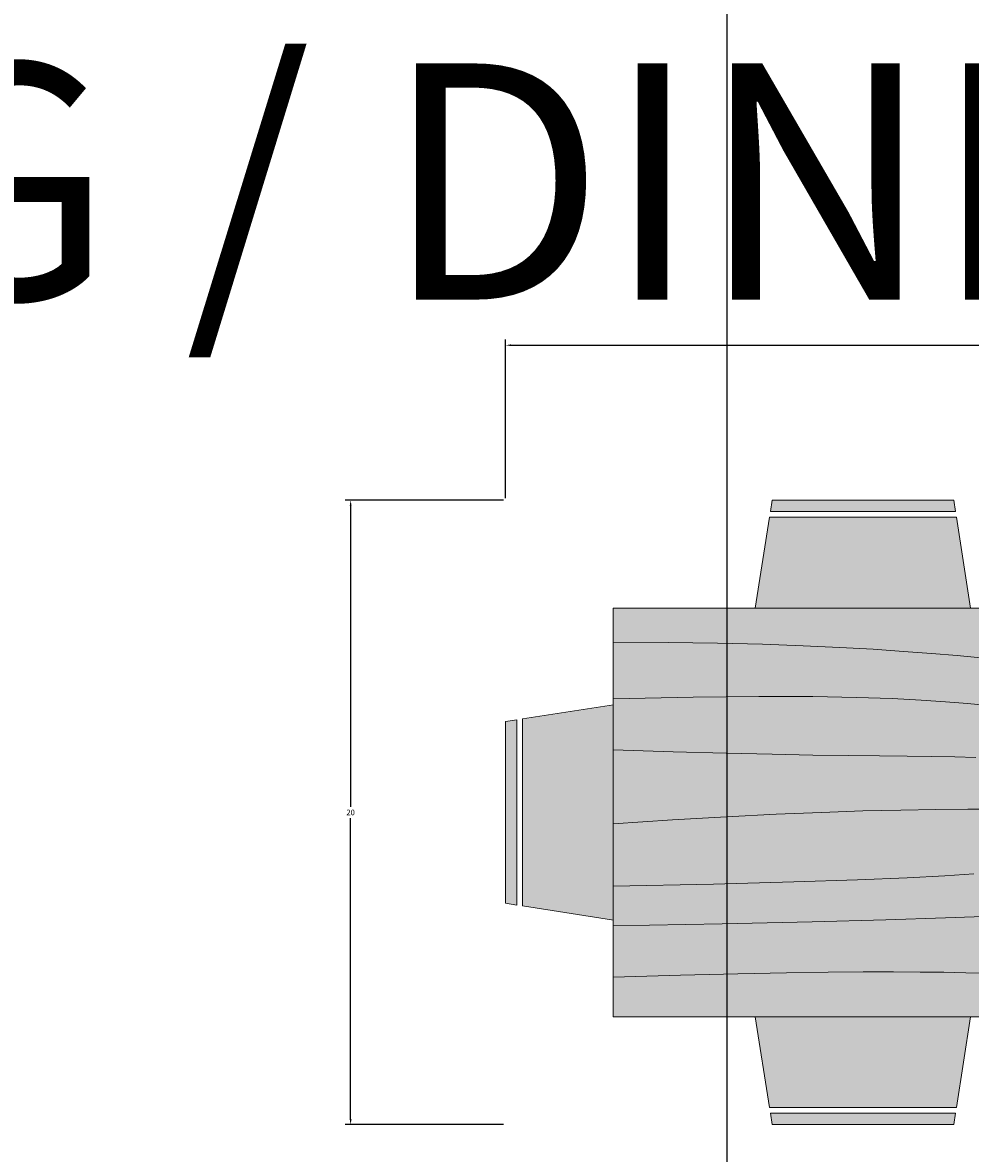
# Model space of a CAD drawing. Units: inches. Extents: x 857 to 1111, y 424 to 822.
# Tile 5 of 9: x 1031 to 1062, y 600 to 636. Entities that reach past the tile are written whole.
import ezdxf

# ---------------------------------------------------------------- set-up
doc = ezdxf.new("R2010")
doc.units = ezdxf.units.IN
for name, color, linetype, lineweight in [('A-ANNO-DIMS', 2, 'Continuous', 18), ('A-AREA-IDEN', 7, 'Continuous', 25), ('A-FURN', 8, 'Continuous', 18), ('A-FURN-PATT', 9, 'Continuous', 13)]:
    doc.layers.add(name, color=color, linetype=linetype, lineweight=lineweight)
doc.styles.get("Standard").update_dxf_attribs({"font": 'arial.ttf'})
doc.dimstyles.get("Standard").update_dxf_attribs({"dimtxt": 0.18, "dimasz": 0.18, "dimexe": 0.18, "dimexo": 0.0625, "dimgap": 0.09, "dimtad": 0, "dimtih": 1, "dimtoh": 1, "dimdec": 4, "dimzin": 0, "dimdsep": 46, "dimtxsty": 'Standard', "dimcen": 0.09, "dimadec": 0, "dimazin": 0, "dimtfac": 1, "dimtdec": 4, "dimtofl": 0, "dimtmove": 0, "dimatfit": 3, "dimfxl": 1, "dimtolj": 1, "dimtzin": 0, "dimarcsym": 0})

# ---------------------------------------------------------------- blocks, each defined once
blk = doc.blocks.new('Dining Set - 36 x 72 in.')
for p, q in [((-22, 27.5), (-22.1562, 26.50042)), ((-22, 27.5), (-6, 27.5)), ((-5.8437, 26.49966), (-6, 27.5)), ((-22.2343, 26.00059), (-23.4847, 17.99762)), ((-22.2304, 26), (-5.7608, 26)), ((-5.8416, 26.5), (-22.1534, 26.5)), ((-4.5152, 17.99762), (-5.7655, 25.99926)), ((36, 18), (-36, 18)), ((-36, 18), (-36, -18)), ((-44.0006, 8.23428), (-35.9976, 9.48474)), ((-45.5, 8), (-44.5004, 8.15617)), ((-45.5, 8), (-45.5, -8)), ((-44.5, -8.15843), (-44.5, 8.15338)), ((-44, 8.23041), (-44, -8.23915)), ((-44.4997, -8.15631), (-45.5, -8)), ((-35.9976, -9.48476), (-43.9993, -8.2345)), ((-36, -18), (36, -18)), ((-22.2343, -26.0006), (-23.4847, -17.99762)), ((-4.5152, -17.99762), (-5.7655, -25.99928)), ((-22.2304, -26), (-5.7608, -26)), ((-22, -27.5), (-22.1562, -26.50044)), ((-5.8416, -26.5), (-22.1534, -26.5)), ((-5.8437, -26.49967), (-6, -27.5)), ((-22, -27.5), (-6, -27.5))]:
    blk.add_line(p, q)
for points in [[(-36, 15), (-31.1772, 14.97754), (-26.8079, 14.91406), (-22.8538, 14.81543), (-19.276, 14.6875), (-16.0362, 14.53613), (-13.0957, 14.36718), (-10.4159, 14.18652), (-7.9583, 14), (-5.6904, 13.81315), (-3.6035, 13.63021)], [(-36, 10), (-28.9766, 10.14274), (-23.1725, 10.20442), (-18.4241, 10.19775), (-14.5677, 10.13541), (-11.4399, 10.03011), (-8.877, 9.89453), (-6.7154, 9.74137), (-4.7917, 9.58333), (-2.9698, 9.43082)], [(-36, 5.5), (-30.7157, 5.3348), (-26.069, 5.20963), (-21.9946, 5.11767), (-18.4271, 5.05208), (-15.3009, 5.00602), (-12.5508, 4.97265), (-10.1112, 4.94515), (-7.9167, 4.91666), (-5.909, 4.88167), (-4.0586, 4.83984)], [(-36, -1), (-30.7915, -0.6591), (-26.0195, -0.38216), (-21.6519, -0.16284), (-17.6563, 0.00521), (-14.0005, 0.12833), (-10.6523, 0.21289), (-7.5796, 0.26522), (-4.75, 0.29166), (-2.134, 0.29793)], [(-36, -6.5), (-27.1843, -6.31267), (-20.084, -6.1263), (-14.469, -5.9419), (-10.1094, -5.76042), (-6.7752, -5.58285), (-4.2363, -5.41016)], [(-36, -10), (-26.4022, -9.81299), (-18.4675, -9.62891), (-11.9839, -9.45069), (-6.7396, -9.28125), (-2.5226, -9.12354)], [(-36, -14.5), (-30.0881, -14.33513), (-25.0332, -14.21224), (-20.7312, -14.12647), (-17.0781, -14.07292), (-13.97, -14.04671), (-11.3027, -14.04297), (-8.9724, -14.05681), (-6.875, -14.08334), (-4.9224, -14.11833), (-3.0905, -14.16016)]]:
    blk.add_lwpolyline(points)
blk = doc.blocks.new('*D30')
at = {"layer": 'A-ANNO-DIMS', "color": 0, "lineweight": -2, "transparency": 16777216}
for p, q in [((1046.887, 621.08), (1046.887, 626.158)), ((1079.951, 621.08), (1079.951, 626.158)), ((1047.067, 625.978), (1062.45, 625.978)), ((1079.771, 625.978), (1064.388, 625.978))]:
    blk.add_line(p, q, dxfattribs=at)
at = {"layer": 'A-ANNO-DIMS', "color": 0, "transparency": 16777216}
for points in [[(1047.067, 626.008), (1047.067, 625.948), (1046.887, 625.978)], [(1079.771, 626.008), (1079.771, 625.948), (1079.951, 625.978)]]:
    blk.add_solid(points, dxfattribs=at)
at = {"layer": 'Defpoints', "color": 0, "transparency": 16777216}
for p in [(1079.951, 625.978), (1046.887, 621.018), (1079.951, 621.018)]:
    blk.add_point(p, dxfattribs=at)
at = {"layer": 'A-ANNO-DIMS', "color": 0, "transparency": 16777216, "insert": (1063.419, 625.978), "char_height": 0.18, "attachment_point": 5}
blk.add_mtext('\\A1;DINING SET 33', dxfattribs=at)
blk = doc.blocks.new('*D31')
at = {"layer": 'A-ANNO-DIMS', "color": 0, "lineweight": -2, "transparency": 16777216}
for p, q in [((1046.824, 621.018), (1041.747, 621.018)), ((1041.927, 620.838), (1041.927, 611.208)), ((1041.927, 601.214), (1041.927, 610.844)), ((1046.824, 601.034), (1041.747, 601.034))]:
    blk.add_line(p, q, dxfattribs=at)
at = {"layer": 'A-ANNO-DIMS', "color": 0, "transparency": 16777216}
for points in [[(1041.897, 620.838), (1041.957, 620.838), (1041.927, 621.018)], [(1041.897, 601.214), (1041.957, 601.214), (1041.927, 601.034)]]:
    blk.add_solid(points, dxfattribs=at)
at = {"layer": 'Defpoints', "color": 0, "transparency": 16777216}
for p in [(1041.927, 621.018), (1046.887, 621.018), (1046.887, 601.034)]:
    blk.add_point(p, dxfattribs=at)
at = {"layer": 'A-ANNO-DIMS', "color": 0, "transparency": 16777216, "insert": (1041.927, 611.026), "char_height": 0.18, "attachment_point": 5}
blk.add_mtext('\\A1;20', dxfattribs=at)
blk = doc.blocks.new('*D55')
at = {"layer": 'A-ANNO-DIMS', "color": 0, "lineweight": -2, "transparency": 16777216}
for p, q in [((1053.972, 717.294), (1053.972, 423.627)), ((1083.137, 717.294), (1083.137, 423.627)), ((1054.152, 423.807), (1068.088, 423.807)), ((1082.957, 423.807), (1069.02, 423.807))]:
    blk.add_line(p, q, dxfattribs=at)
at = {"layer": 'A-ANNO-DIMS', "color": 0, "transparency": 16777216}
for points in [[(1054.152, 423.837), (1054.152, 423.777), (1053.972, 423.807)], [(1082.957, 423.837), (1082.957, 423.777), (1083.137, 423.807)]]:
    blk.add_solid(points, dxfattribs=at)
at = {"layer": 'Defpoints', "color": 0, "transparency": 16777216}
for p in [(1053.972, 717.357), (1083.137, 717.357), (1083.137, 423.807)]:
    blk.add_point(p, dxfattribs=at)
at = {"layer": 'A-ANNO-DIMS', "color": 0, "transparency": 16777216, "insert": (1068.554, 423.807), "char_height": 0.18, "attachment_point": 5}
blk.add_mtext('\\A1;29.165', dxfattribs=at)
blk = doc.blocks.new('*D56')
at = {"layer": 'A-ANNO-DIMS', "color": 0, "lineweight": -2, "transparency": 16777216}
for p, q in [((924.77, 717.294), (924.77, 423.627)), ((1053.972, 717.294), (1053.972, 423.627)), ((924.95, 423.807), (988.986, 423.807)), ((1053.792, 423.807), (989.755, 423.807))]:
    blk.add_line(p, q, dxfattribs=at)
at = {"layer": 'A-ANNO-DIMS', "color": 0, "transparency": 16777216}
for points in [[(924.95, 423.837), (924.95, 423.777), (924.77, 423.807)], [(1053.792, 423.837), (1053.792, 423.777), (1053.972, 423.807)]]:
    blk.add_solid(points, dxfattribs=at)
at = {"layer": 'Defpoints', "color": 0, "transparency": 16777216}
for p in [(924.77, 717.357), (1053.972, 717.357), (1053.972, 423.807)]:
    blk.add_point(p, dxfattribs=at)
at = {"layer": 'A-ANNO-DIMS', "color": 0, "transparency": 16777216, "insert": (989.371, 423.807), "char_height": 0.18, "attachment_point": 5}
blk.add_mtext('\\A1;129.2', dxfattribs=at)

msp = doc.modelspace()

# ---------------------------------------------------------------- hatches: boundary and pattern name
at = {"layer": 'A-FURN-PATT'}
h = msp.add_hatch(color=256, dxfattribs=at)
h.dxf.hatch_style = 1
h.paths.add_polyline_path([(1071.4125, 621.0178), (1065.599, 621.0178), (1065.5422, 620.6545), (1071.4693, 620.6545)])
h.paths.add_polyline_path([(1071.4977, 620.4728), (1065.5138, 620.4728), (1065.0596, 617.566), (1071.9519, 617.566)])
h.paths.add_polyline_path([(1061.324, 620.4728), (1055.3401, 620.4728), (1054.8859, 617.566), (1061.7782, 617.566)])
h.paths.add_polyline_path([(1061.2388, 621.0178), (1055.4253, 621.0178), (1055.3685, 620.6545), (1061.2956, 620.6545)])
h.paths.add_polyline_path([(1050.3384, 614.4719), (1047.4316, 614.0177), (1047.4316, 608.0338), (1050.3384, 607.5797)])
h.paths.add_polyline_path([(1047.25, 613.9893), (1046.8866, 613.9326), (1046.8866, 608.119), (1047.25, 608.0622)])
h.paths.add_polyline_path([(1061.7782, 604.4855), (1054.8859, 604.4855), (1055.3401, 601.5788), (1061.324, 601.5788)])
h.paths.add_polyline_path([(1061.2956, 601.3971), (1055.3685, 601.3971), (1055.4253, 601.0337), (1061.2388, 601.0337)])
h.paths.add_polyline_path([(1071.4693, 601.3971), (1065.5422, 601.3971), (1065.599, 601.0337), (1071.4125, 601.0337)])
h.paths.add_polyline_path([(1071.9519, 604.4855), (1065.0596, 604.4855), (1065.5138, 601.5788), (1071.4977, 601.5788)])
h.paths.add_polyline_path([(1079.4062, 614.0177), (1076.4994, 614.4719), (1076.4994, 607.5797), (1079.4062, 608.0338)])
h.paths.add_polyline_path([(1079.9512, 613.9326), (1079.5878, 613.9893), (1079.5878, 608.0622), (1079.9512, 608.119)])
h = msp.add_hatch(color=256, dxfattribs=at)
h.dxf.hatch_style = 1
h.paths.add_polyline_path([(1066.6626, 616.5198), (1066.6356, 616.5664), (1066.6135, 616.6122), (1066.5982, 616.6577), (1066.5911, 616.703), (1066.5925, 616.7476), (1066.6024, 616.7907), (1066.6209, 616.8318), (1066.6478, 616.87), (1066.6833, 616.9046), (1066.7273, 616.935), (1066.7798, 616.9605), (1066.8412, 616.9803), (1066.9133, 616.9945), (1066.9981, 617.003), (1067.0978, 617.0059), (1067.2145, 617.003), (1067.3504, 616.9945), (1067.5076, 616.9803), (1067.6882, 616.9605), (1067.8947, 616.935), (1068.1313, 616.9042), (1068.4022, 616.8684), (1068.712, 616.828), (1069.0651, 616.7833), (1069.4659, 616.7348), (1069.9189, 616.6827), (1070.4285, 616.6274), (1070.9979, 616.5692), (1071.6261, 616.5086), (1072.3108, 616.4459), (1073.0495, 616.3814), (1073.84, 616.3154), (1074.6801, 616.2484), (1075.5673, 616.1807), (1076.4994, 616.1126), (1076.4994, 617.566), (1050.3384, 617.566), (1050.3384, 616.476), (1052.0907, 616.4678), (1053.6783, 616.4448), (1055.115, 616.4089), (1056.415, 616.3624), (1057.5922, 616.3074), (1058.6606, 616.2461), (1059.6343, 616.1804), (1060.5273, 616.1126), (1061.3513, 616.0448), (1062.1096, 615.9783), (1062.8029, 615.9146), (1063.4322, 615.8553), (1063.9982, 615.8016), (1064.5021, 615.755), (1064.9445, 615.7169), (1065.3265, 615.6887), (1065.6496, 615.6716), (1065.9188, 615.6651), (1066.1397, 615.6685), (1066.3181, 615.6812), (1066.4596, 615.7023), (1066.5698, 615.7313), (1066.6545, 615.7674), (1066.7193, 615.8099), (1066.7691, 615.8579), (1066.8059, 615.9106), (1066.8305, 615.9669), (1066.8442, 616.0256), (1066.8479, 616.0857), (1066.8428, 616.1462), (1066.8298, 616.206), (1066.8101, 616.264), (1066.7849, 616.3194), (1066.7557, 616.3724), (1066.7244, 616.4232), (1066.6928, 616.4722)])
h.paths.add_polyline_path([(1069.2432, 615.5925), (1069.2973, 615.6433), (1069.3634, 615.6885), (1069.4406, 615.7266), (1069.5277, 615.7562), (1069.6237, 615.7758), (1069.7275, 615.7841), (1069.838, 615.7796), (1069.9553, 615.7613), (1070.0833, 615.7301), (1070.2274, 615.6872), (1070.3925, 615.6339), (1070.5839, 615.5713), (1070.8067, 615.5007), (1071.0661, 615.4234), (1071.3671, 615.3405), (1071.7162, 615.2528), (1072.1243, 615.1581), (1072.6038, 615.0539), (1073.1668, 614.9374), (1073.8257, 614.8061), (1074.5925, 614.6571), (1075.4797, 614.488), (1076.4994, 614.2959), (1076.4994, 616.1126), (1075.5673, 616.1807), (1074.6801, 616.2484), (1073.84, 616.3154), (1073.0495, 616.3814), (1072.3108, 616.4459), (1071.6261, 616.5086), (1070.9979, 616.5692), (1070.4285, 616.6274), (1069.9189, 616.6827), (1069.4659, 616.7348), (1069.0651, 616.7833), (1068.712, 616.828), (1068.4022, 616.8684), (1068.1313, 616.9042), (1067.8947, 616.935), (1067.6882, 616.9605), (1067.5076, 616.9803), (1067.3504, 616.9945), (1067.2145, 617.003), (1067.0978, 617.0059), (1066.9981, 617.003), (1066.9133, 616.9945), (1066.8412, 616.9803), (1066.7798, 616.9605), (1066.7273, 616.935), (1066.6833, 616.9046), (1066.6478, 616.87), (1066.6209, 616.8318), (1066.6024, 616.7907), (1066.5925, 616.7476), (1066.5911, 616.703), (1066.5982, 616.6577), (1066.6135, 616.6122), (1066.6356, 616.5664), (1066.6626, 616.5198), (1066.6928, 616.4722), (1066.7244, 616.4232), (1066.7557, 616.3724), (1066.7849, 616.3194), (1066.8101, 616.264), (1066.8298, 616.206), (1066.8428, 616.1462), (1066.8479, 616.0857), (1066.8442, 616.0256), (1066.8305, 615.9669), (1066.8059, 615.9106), (1066.7691, 615.8579), (1066.7193, 615.8099), (1066.6545, 615.7674), (1066.5698, 615.7313), (1066.4596, 615.7023), (1066.3181, 615.6812), (1066.1397, 615.6685), (1065.9188, 615.6651), (1065.6496, 615.6716), (1065.3265, 615.6887), (1064.9445, 615.7169), (1064.5021, 615.755), (1063.9982, 615.8016), (1063.4322, 615.8553), (1062.8029, 615.9146), (1062.1096, 615.9783), (1061.3513, 616.0448), (1060.5273, 616.1126), (1059.6343, 616.1804), (1058.6606, 616.2461), (1057.5922, 616.3074), (1056.415, 616.3624), (1055.115, 616.4089), (1053.6783, 616.4448), (1052.0907, 616.4678), (1050.3384, 616.476), (1050.3384, 614.6593), (1052.8903, 614.7111), (1054.9992, 614.7335), (1056.7245, 614.7311), (1058.1258, 614.7085), (1059.2622, 614.6702), (1060.1935, 614.6209), (1060.9789, 614.5653), (1061.6778, 614.5079), (1062.3398, 614.4524), (1062.9739, 614.3995), (1063.5793, 614.3487), (1064.155, 614.2997), (1064.7003, 614.2521), (1065.2141, 614.2055), (1065.6956, 614.1597), (1066.144, 614.1142), (1066.5586, 614.069), (1066.9402, 614.0248), (1067.2899, 613.9828), (1067.6087, 613.9439), (1067.8978, 613.9093), (1068.158, 613.88), (1068.3906, 613.8572), (1068.5966, 613.8417), (1068.7772, 613.8346), (1068.9344, 613.8356), (1069.0703, 613.8444), (1069.187, 613.8606), (1069.2867, 613.884), (1069.3715, 613.9141), (1069.4436, 613.9506), (1069.5049, 613.9931), (1069.5574, 614.0413), (1069.601, 614.0944), (1069.6354, 614.1517), (1069.6601, 614.2126), (1069.675, 614.2764), (1069.6795, 614.3423), (1069.6734, 614.4096), (1069.6564, 614.4776), (1069.6283, 614.5457), (1069.5911, 614.6138), (1069.5467, 614.682), (1069.4974, 614.7501), (1069.4452, 614.8182), (1069.3923, 614.8863), (1069.3409, 614.9545), (1069.293, 615.0226), (1069.2506, 615.0907), (1069.2149, 615.1584), (1069.1871, 615.2254), (1069.1681, 615.2913), (1069.159, 615.3558), (1069.161, 615.4186), (1069.175, 615.4792), (1069.2022, 615.5373)])
h.paths.add_polyline_path([(1076.4994, 614.2959), (1075.4797, 614.488), (1074.5925, 614.6571), (1073.8257, 614.8061), (1073.1668, 614.9374), (1072.6038, 615.0539), (1072.1243, 615.1581), (1071.7162, 615.2528), (1071.3671, 615.3405), (1071.0661, 615.4234), (1070.8067, 615.5007), (1070.5839, 615.5713), (1070.3925, 615.6339), (1070.2274, 615.6872), (1070.0833, 615.7301), (1069.9553, 615.7613), (1069.838, 615.7796), (1069.7275, 615.7841), (1069.6237, 615.7758), (1069.5277, 615.7562), (1069.4406, 615.7266), (1069.3634, 615.6885), (1069.2973, 615.6433), (1069.2432, 615.5925), (1069.2022, 615.5373), (1069.175, 615.4792), (1069.161, 615.4186), (1069.159, 615.3558), (1069.1681, 615.2913), (1069.1871, 615.2254), (1069.2149, 615.1584), (1069.2506, 615.0907), (1069.293, 615.0226), (1069.3409, 614.9545), (1069.3923, 614.8863), (1069.4452, 614.8182), (1069.4974, 614.7501), (1069.5467, 614.682), (1069.5911, 614.6138), (1069.6283, 614.5457), (1069.6564, 614.4776), (1069.6734, 614.4096), (1069.6795, 614.3423), (1069.675, 614.2764), (1069.6601, 614.2126), (1069.6354, 614.1517), (1069.601, 614.0944), (1069.5574, 614.0413), (1069.5049, 613.9931), (1069.4436, 613.9506), (1069.3715, 613.9141), (1069.2867, 613.884), (1069.187, 613.8606), (1069.0703, 613.8444), (1068.9344, 613.8356), (1068.7772, 613.8346), (1068.5966, 613.8417), (1068.3906, 613.8572), (1068.158, 613.88), (1067.8978, 613.9093), (1067.6087, 613.9439), (1067.2899, 613.9828), (1066.9402, 614.0248), (1066.5586, 614.069), (1066.144, 614.1142), (1065.6956, 614.1597), (1065.2141, 614.2055), (1064.7003, 614.2521), (1064.155, 614.2997), (1063.5793, 614.3487), (1062.9739, 614.3995), (1062.3398, 614.4524), (1061.6778, 614.5079), (1060.9789, 614.5653), (1060.1935, 614.6209), (1059.2622, 614.6702), (1058.1258, 614.7085), (1056.7245, 614.7311), (1054.9992, 614.7335), (1052.8903, 614.7111), (1050.3384, 614.6593), (1050.3384, 613.0242), (1052.2584, 612.9642), (1053.9468, 612.9187), (1055.4272, 612.8853), (1056.7235, 612.8614), (1057.8594, 612.8447), (1058.8586, 612.8326), (1059.745, 612.8226), (1060.5424, 612.8122), (1061.2719, 612.7995), (1061.9442, 612.7843), (1062.5676, 612.767), (1063.1502, 612.7479), (1063.7001, 612.7274), (1064.2255, 612.7058), (1064.7347, 612.6835), (1065.2356, 612.6608), (1065.7345, 612.6383), (1066.2292, 612.6164), (1066.7153, 612.5959), (1067.1886, 612.5776), (1067.6449, 612.5621), (1068.0799, 612.5501), (1068.4894, 612.5425), (1068.8691, 612.5397), (1069.2157, 612.5426), (1069.53, 612.5511), (1069.8138, 612.5653), (1070.0689, 612.5851), (1070.297, 612.6107), (1070.4999, 612.6419), (1070.6794, 612.6788), (1070.8372, 612.7214), (1070.9754, 612.7695), (1071.0965, 612.8222), (1071.2034, 612.8784), (1071.299, 612.9371), (1071.386, 612.9973), (1071.4674, 613.0578), (1071.5459, 613.1176), (1071.6245, 613.1756), (1071.7056, 613.2308), (1071.7905, 613.2825), (1071.8805, 613.3299), (1071.9765, 613.3724), (1072.0796, 613.4092), (1072.1908, 613.4396), (1072.3113, 613.4629), (1072.442, 613.4784), (1072.5838, 613.4855), (1072.7358, 613.4845), (1072.8971, 613.4757), (1073.0665, 613.4595), (1073.243, 613.4361), (1073.4256, 613.406), (1073.6131, 613.3695), (1073.8046, 613.327), (1074.0011, 613.2785), (1074.2129, 613.2229), (1074.4523, 613.1588), (1074.7318, 613.0847), (1075.0639, 612.9994), (1075.4609, 612.9012), (1075.9353, 612.7888), (1076.4994, 612.6608)])
h.paths.add_polyline_path([(1076.4994, 612.6608), (1075.9353, 612.7888), (1075.4609, 612.9012), (1075.0639, 612.9994), (1074.7318, 613.0847), (1074.4523, 613.1588), (1074.2129, 613.2229), (1074.0011, 613.2785), (1073.8046, 613.327), (1073.6131, 613.3695), (1073.4256, 613.406), (1073.243, 613.4361), (1073.0665, 613.4595), (1072.8971, 613.4757), (1072.7358, 613.4845), (1072.5838, 613.4855), (1072.442, 613.4784), (1072.3113, 613.4629), (1072.1908, 613.4396), (1072.0796, 613.4092), (1071.9765, 613.3724), (1071.8805, 613.3299), (1071.7905, 613.2825), (1071.7056, 613.2308), (1071.6245, 613.1756), (1071.5459, 613.1176), (1071.4674, 613.0578), (1071.386, 612.9973), (1071.299, 612.9371), (1071.2034, 612.8784), (1071.0965, 612.8222), (1070.9754, 612.7695), (1070.8372, 612.7214), (1070.6794, 612.6788), (1070.4999, 612.6419), (1070.297, 612.6107), (1070.0689, 612.5851), (1069.8138, 612.5653), (1069.53, 612.5511), (1069.2157, 612.5426), (1068.8691, 612.5397), (1068.4894, 612.5425), (1068.0799, 612.5501), (1067.6449, 612.5621), (1067.1886, 612.5776), (1066.7153, 612.5959), (1066.2292, 612.6164), (1065.7345, 612.6383), (1065.2356, 612.6608), (1064.7347, 612.6835), (1064.2255, 612.7058), (1063.7001, 612.7274), (1063.1502, 612.7479), (1062.5676, 612.767), (1061.9442, 612.7843), (1061.2719, 612.7995), (1060.5424, 612.8122), (1059.745, 612.8226), (1058.8586, 612.8326), (1057.8594, 612.8447), (1056.7235, 612.8614), (1055.4272, 612.8853), (1053.9468, 612.9187), (1052.2584, 612.9642), (1050.3384, 613.0242), (1050.3384, 610.6624), (1052.2309, 610.7863), (1053.9648, 610.8869), (1055.5517, 610.9666), (1057.0035, 611.0277), (1058.3319, 611.0724), (1059.5484, 611.1031), (1060.6649, 611.1222), (1061.693, 611.1318), (1062.6435, 611.134), (1063.5235, 611.1301), (1064.3388, 611.1208), (1065.0956, 611.1072), (1065.7999, 611.0899), (1066.4577, 611.07), (1067.075, 611.0483), (1067.6579, 611.0258), (1068.2114, 611.0033), (1068.7361, 610.9818), (1069.2318, 610.9624), (1069.698, 610.9463), (1070.1344, 610.9344), (1070.5406, 610.9279), (1070.9163, 610.9277), (1071.2612, 610.9349), (1071.5753, 610.9503), (1071.8615, 610.9728), (1072.1228, 611.0009), (1072.3625, 611.0334), (1072.5838, 611.0686), (1072.7898, 611.1053), (1072.9837, 611.1419), (1073.1687, 611.1772), (1073.3479, 611.2097), (1073.5235, 611.2387), (1073.6978, 611.2634), (1073.8727, 611.2832), (1074.0505, 611.2972), (1074.2332, 611.3049), (1074.423, 611.3055), (1074.6221, 611.2983), (1074.8312, 611.283), (1075.0458, 611.2609), (1075.26, 611.2339), (1075.468, 611.2037), (1075.664, 611.172), (1075.842, 611.1407), (1075.9963, 611.1116), (1076.1209, 611.0863), (1076.2123, 611.0664), (1076.2758, 611.0513), (1076.3192, 611.0406), (1076.3499, 611.0334), (1076.3756, 611.029), (1076.4041, 611.0267), (1076.4428, 611.0259), (1076.4994, 611.0258)])
h.paths.add_polyline_path([(1076.4994, 611.0258), (1076.4428, 611.0259), (1076.4041, 611.0267), (1076.3756, 611.029), (1076.3499, 611.0334), (1076.3192, 611.0406), (1076.2758, 611.0513), (1076.2123, 611.0664), (1076.1209, 611.0863), (1075.9963, 611.1116), (1075.842, 611.1407), (1075.664, 611.172), (1075.468, 611.2037), (1075.26, 611.2339), (1075.0458, 611.2609), (1074.8312, 611.283), (1074.6221, 611.2983), (1074.423, 611.3055), (1074.2332, 611.3049), (1074.0505, 611.2972), (1073.8727, 611.2832), (1073.6978, 611.2634), (1073.5235, 611.2387), (1073.3479, 611.2097), (1073.1687, 611.1772), (1072.9837, 611.1419), (1072.7898, 611.1053), (1072.5838, 611.0686), (1072.3625, 611.0334), (1072.1228, 611.0009), (1071.8615, 610.9728), (1071.5753, 610.9503), (1071.2612, 610.9349), (1070.9163, 610.9277), (1070.5406, 610.9279), (1070.1344, 610.9344), (1069.698, 610.9463), (1069.2318, 610.9624), (1068.7361, 610.9818), (1068.2114, 611.0033), (1067.6579, 611.0258), (1067.075, 611.0483), (1066.4577, 611.07), (1065.7999, 611.0899), (1065.0956, 611.1072), (1064.3388, 611.1208), (1063.5235, 611.1301), (1062.6435, 611.134), (1061.693, 611.1318), (1060.6649, 611.1222), (1059.5484, 611.1031), (1058.3319, 611.0724), (1057.0035, 611.0277), (1055.5517, 610.9666), (1053.9648, 610.8869), (1052.2309, 610.7863), (1050.3384, 610.6624), (1050.3384, 608.664), (1053.5416, 608.7321), (1056.1214, 608.7998), (1058.1616, 608.8668), (1059.7457, 608.9328), (1060.9571, 608.9973), (1061.8796, 609.06), (1062.5967, 609.1206), (1063.1918, 609.1788), (1063.7353, 609.2341), (1064.2442, 609.2866), (1064.7223, 609.3363), (1065.1732, 609.3832), (1065.6006, 609.4272), (1066.0085, 609.4683), (1066.4003, 609.5066), (1066.7798, 609.5421), (1067.1506, 609.5746), (1067.515, 609.6036), (1067.8752, 609.6283), (1068.2332, 609.6481), (1068.5913, 609.6622), (1068.9514, 609.6699), (1069.3158, 609.6704), (1069.6866, 609.6632), (1070.0649, 609.6478), (1070.4479, 609.6249), (1070.8315, 609.5956), (1071.2119, 609.561), (1071.5853, 609.5222), (1071.9476, 609.4801), (1072.2951, 609.436), (1072.6237, 609.3907), (1072.9308, 609.3453), (1073.2181, 609.3001), (1073.4889, 609.2553), (1073.7459, 609.2109), (1073.9923, 609.1673), (1074.2311, 609.1246), (1074.4652, 609.0829), (1074.6978, 609.0425), (1074.9311, 609.004), (1075.1645, 608.9699), (1075.3969, 608.9433), (1075.627, 608.9271), (1075.8535, 608.9244), (1076.0752, 608.9382), (1076.291, 608.9715), (1076.4994, 609.0274)])
h.paths.add_polyline_path([(1076.4994, 609.0274), (1076.291, 608.9715), (1076.0752, 608.9382), (1075.8535, 608.9244), (1075.627, 608.9271), (1075.3969, 608.9433), (1075.1645, 608.9699), (1074.9311, 609.004), (1074.6978, 609.0425), (1074.4652, 609.0829), (1074.2311, 609.1246), (1073.9923, 609.1673), (1073.7459, 609.2109), (1073.4889, 609.2553), (1073.2181, 609.3001), (1072.9308, 609.3453), (1072.6237, 609.3907), (1072.2951, 609.436), (1071.9476, 609.4801), (1071.5853, 609.5222), (1071.2119, 609.561), (1070.8315, 609.5956), (1070.4479, 609.6249), (1070.0649, 609.6478), (1069.6866, 609.6632), (1069.3158, 609.6704), (1068.9514, 609.6699), (1068.5913, 609.6622), (1068.2332, 609.6481), (1067.8752, 609.6283), (1067.515, 609.6036), (1067.1506, 609.5746), (1066.7798, 609.5421), (1066.4003, 609.5066), (1066.0085, 609.4683), (1065.6006, 609.4272), (1065.1732, 609.3832), (1064.7223, 609.3363), (1064.2442, 609.2866), (1063.7353, 609.2341), (1063.1918, 609.1788), (1062.5967, 609.1206), (1061.8796, 609.06), (1060.9571, 608.9973), (1059.7457, 608.9328), (1058.1616, 608.8668), (1056.1214, 608.7998), (1053.5416, 608.7321), (1050.3384, 608.664), (1050.3384, 607.3923), (1053.8257, 607.4603), (1056.7088, 607.5272), (1059.0646, 607.5919), (1060.9701, 607.6535), (1062.5023, 607.7108), (1063.7382, 607.7628), (1064.7549, 607.8084), (1065.6292, 607.8465), (1066.4262, 607.8764), (1067.1621, 607.8985), (1067.8413, 607.9136), (1068.4679, 607.9222), (1069.0463, 607.9252), (1069.5806, 607.9231), (1070.0753, 607.9169), (1070.5345, 607.9071), (1070.9626, 607.8943), (1071.3647, 607.8789), (1071.7464, 607.861), (1072.1127, 607.8408), (1072.4692, 607.8185), (1072.821, 607.7942), (1073.1735, 607.7682), (1073.5321, 607.7405), (1073.9005, 607.7116), (1074.2767, 607.6826), (1074.6572, 607.6546), (1075.0384, 607.6289), (1075.4168, 607.6067), (1075.7888, 607.5894), (1076.1508, 607.578), (1076.4994, 607.574)])
h.paths.add_polyline_path([(1076.4994, 606.3023), (1074.9834, 606.1184), (1073.6879, 605.9728), (1072.5866, 605.8608), (1071.6529, 605.7781), (1070.8604, 605.7202), (1070.1827, 605.6827), (1069.5934, 605.6612), (1069.0659, 605.6513), (1068.5771, 605.649), (1068.1166, 605.6529), (1067.677, 605.6622), (1067.2511, 605.6759), (1066.8315, 605.6931), (1066.4111, 605.713), (1065.9824, 605.7347), (1065.5384, 605.7573), (1065.0724, 605.7799), (1064.5806, 605.8022), (1064.0601, 605.8238), (1063.5078, 605.8443), (1062.9208, 605.8634), (1062.296, 605.8807), (1061.6304, 605.8959), (1060.9209, 605.9086), (1060.1588, 605.9183), (1059.3121, 605.9233), (1058.3429, 605.922), (1057.2136, 605.9124), (1055.8863, 605.893), (1054.3232, 605.8618), (1052.4865, 605.8172), (1050.3384, 605.7573), (1050.3384, 604.4855), (1076.4994, 604.4855)])
h.paths.add_polyline_path([(1076.4994, 607.574), (1076.1508, 607.578), (1075.7888, 607.5894), (1075.4168, 607.6067), (1075.0384, 607.6289), (1074.6572, 607.6546), (1074.2767, 607.6826), (1073.9005, 607.7116), (1073.5321, 607.7405), (1073.1735, 607.7682), (1072.821, 607.7942), (1072.4692, 607.8185), (1072.1127, 607.8408), (1071.7464, 607.861), (1071.3647, 607.8789), (1070.9626, 607.8943), (1070.5345, 607.9071), (1070.0753, 607.9169), (1069.5806, 607.9231), (1069.0463, 607.9252), (1068.4679, 607.9222), (1067.8413, 607.9136), (1067.1621, 607.8985), (1066.4262, 607.8764), (1065.6292, 607.8465), (1064.7549, 607.8084), (1063.7382, 607.7628), (1062.5023, 607.7108), (1060.9701, 607.6535), (1059.0646, 607.5919), (1056.7088, 607.5272), (1053.8257, 607.4603), (1050.3384, 607.3923), (1050.3384, 605.7573), (1052.4865, 605.8172), (1054.3232, 605.8618), (1055.8863, 605.893), (1057.2136, 605.9124), (1058.3429, 605.922), (1059.3121, 605.9233), (1060.1588, 605.9183), (1060.9209, 605.9086), (1061.6304, 605.8959), (1062.296, 605.8807), (1062.9208, 605.8634), (1063.5078, 605.8443), (1064.0601, 605.8238), (1064.5806, 605.8022), (1065.0724, 605.7799), (1065.5384, 605.7573), (1065.9824, 605.7347), (1066.4111, 605.713), (1066.8315, 605.6931), (1067.2511, 605.6759), (1067.677, 605.6622), (1068.1166, 605.6529), (1068.5771, 605.649), (1069.0659, 605.6513), (1069.5934, 605.6612), (1070.1827, 605.6827), (1070.8604, 605.7202), (1071.6529, 605.7781), (1072.5866, 605.8608), (1073.6879, 605.9728), (1074.9834, 606.1184), (1076.4994, 606.3023)])

# ---------------------------------------------------------------- block references
at = {"layer": 'A-FURN', "xscale": 0.3633469118061226, "yscale": 0.3633469118061226, "zscale": 0.3633469118061226}
msp.add_blockref('Dining Set - 36 x 72 in.', (1063.4189, 611.0258), dxfattribs=at)

# ---------------------------------------------------------------- texts
at = {"layer": 'A-AREA-IDEN'}
msp.add_text('LIVING / DINING ', height=7.55928, dxfattribs=at).set_placement((1002.1837, 627.4375))

# ---------------------------------------------------------------- dimensions: what is measured, and where the dimension line sits
at = {"layer": 'A-ANNO-DIMS'}
for base, p1, p2, override, picture, middle in [((1053.9717, 423.8067), (924.7696, 717.3567), (1053.9717, 717.3567), {"dimdec": 1, "dimlfac": 1, "dimrnd": 0, "dimzin": 0, "dimdsep": 46, "dimlunit": 2}, '*D56', (989.3707, 423.8067)), ((1083.1369, 423.8067), (1053.9717, 717.3567), (1083.1369, 717.3567), {"dimdec": 3, "dimlfac": 1, "dimrnd": 0, "dimzin": 0, "dimdsep": 46, "dimlunit": 2}, '*D55', (1068.5543, 423.8067))]:
    dim = msp.add_linear_dim(base=base, p1=p1, p2=p2, dimstyle='Standard', override=override, dxfattribs=at)
    dim.commit()
    dim.dimension.update_dxf_attribs({"geometry": picture, "text_midpoint": middle})
dim = msp.add_linear_dim(base=(1079.9512, 625.9775), p1=(1046.8866, 621.0178), p2=(1079.9512, 621.0178), text='DINING SET <>', dimstyle='Standard', override={"dimdec": 0, "dimlfac": 1, "dimrnd": 0, "dimzin": 0, "dimdsep": 46, "dimlunit": 2}, dxfattribs=at)
dim.commit()
dim.dimension.update_dxf_attribs({"geometry": '*D30', "text_midpoint": (1063.4189, 625.9775)})
dim = msp.add_linear_dim(base=(1041.9269, 621.0178), p1=(1046.8866, 601.0337), p2=(1046.8866, 621.0178), angle=90, dimstyle='Standard', override={"dimdec": 0, "dimlfac": 1, "dimrnd": 0, "dimzin": 0, "dimdsep": 46, "dimlunit": 2}, dxfattribs=at)
dim.commit()
dim.dimension.update_dxf_attribs({"geometry": '*D31', "text_midpoint": (1041.9269, 611.0258)})

doc.saveas('drawing.dxf')
